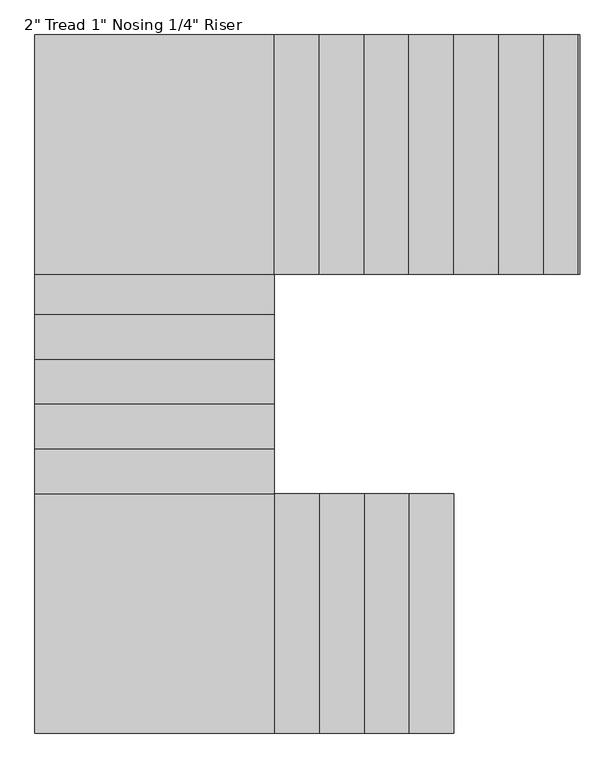
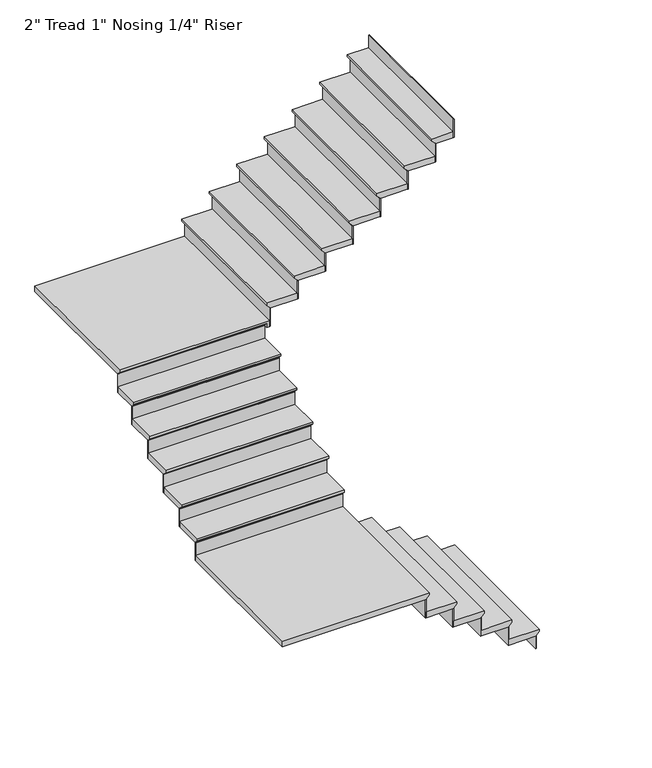
"""IFC4 building model written with IfcOpenShell, lengths in millimetres: stair flight geometry."""

from ifc_helpers import new_model, si_unit, origin, place, context, project, spatial, faceted_brep, source, transform, mapped, element, save


def stair_flight_d9589ae6(model_context):
    return source(origin(), model_context, "Body", "Brep", [
        faceted_brep([(-2683.1105391, -1521.8373761, 12790.5710526), (-2683.1105391, -1521.8373761, 12809.6210526), (-2683.1105391, -2741.0373761, 12809.6210526), (-2683.1105391, -2741.0373761, 12790.5710526), (-2708.5105391, -1521.8373761, 12765.1710526), (-2708.5105391, -2741.0373761, 12765.1710526), (-2937.1105391, -1521.8373761, 12809.6210526), (-2937.1105391, -2741.0373761, 12809.6210526), (-2708.5105391, -2741.0373761, 12758.8210526), (-2937.1105391, -2741.0373761, 12758.8210526), (-2937.1105391, -1521.8373761, 12758.8210526), (-2708.5105391, -1521.8373761, 12758.8210526)], [[[0, 1, 2, 3]], [[4, 0, 3, 5]], [[2, 1, 6, 7]], [[8, 9, 10, 11]], [[2, 7, 9, 8, 5, 3]], [[8, 11, 4, 5]], [[6, 1, 0, 4, 11, 10]], [[7, 6, 10, 9]]]),
        faceted_brep([(-2708.5105391, -1521.8373761, 12758.8210526), (-2708.5105391, -1521.8373761, 12649.2), (-2714.8605391, -1521.8373761, 12649.2), (-2714.8605391, -1521.8373761, 12758.8210526), (-2708.5105391, -2741.0373761, 12758.8210526), (-2714.8605391, -2741.0373761, 12758.8210526), (-2714.8605391, -2741.0373761, 12649.2), (-2708.5105391, -2741.0373761, 12649.2)], [[[0, 1, 2, 3]], [[4, 5, 6, 7]], [[1, 0, 4, 7]], [[2, 1, 7, 6]], [[3, 2, 6, 5]], [[0, 3, 5, 4]]]),
        faceted_brep([(-2937.1105391, -1521.8373761, 12919.2421053), (-2937.1105391, -1521.8373761, 12758.8210526), (-2943.4605391, -1521.8373761, 12758.8210526), (-2943.4605391, -1521.8373761, 12919.2421053), (-2937.1105391, -2741.0373761, 12919.2421053), (-2943.4605391, -2741.0373761, 12919.2421053), (-2943.4605391, -2741.0373761, 12758.8210526), (-2937.1105391, -2741.0373761, 12758.8210526)], [[[0, 1, 2, 3]], [[4, 5, 6, 7]], [[1, 0, 4, 7]], [[2, 1, 7, 6]], [[3, 2, 6, 5]], [[0, 3, 5, 4]]]),
        faceted_brep([(-2911.7105391, -2741.0373761, 12970.0421053), (-2911.7105391, -1521.8373761, 12970.0421053), (-3165.7105391, -1521.8373761, 12970.0421053), (-3165.7105391, -2741.0373761, 12970.0421053), (-2937.1105391, -2741.0373761, 12919.2421053), (-3165.7105391, -2741.0373761, 12919.2421053), (-3165.7105391, -1521.8373761, 12919.2421053), (-2937.1105391, -1521.8373761, 12919.2421053), (-2937.1105391, -2741.0373761, 12925.5921053), (-2911.7105391, -2741.0373761, 12950.9921053), (-2937.1105391, -1521.8373761, 12925.5921053), (-2911.7105391, -1521.8373761, 12950.9921053)], [[[0, 1, 2, 3]], [[4, 5, 6, 7]], [[0, 3, 5, 4, 8, 9]], [[4, 7, 10, 8]], [[2, 1, 11, 10, 7, 6]], [[3, 2, 6, 5]], [[11, 1, 0, 9]], [[10, 11, 9, 8]]]),
        faceted_brep([(-3165.7105391, -1521.8373761, 13079.6631579), (-3165.7105391, -1521.8373761, 12919.2421053), (-3172.0605391, -1521.8373761, 12919.2421053), (-3172.0605391, -1521.8373761, 13079.6631579), (-3165.7105391, -2741.0373761, 13079.6631579), (-3172.0605391, -2741.0373761, 13079.6631579), (-3172.0605391, -2741.0373761, 12919.2421053), (-3165.7105391, -2741.0373761, 12919.2421053)], [[[0, 1, 2, 3]], [[4, 5, 6, 7]], [[1, 0, 4, 7]], [[2, 1, 7, 6]], [[3, 2, 6, 5]], [[0, 3, 5, 4]]]),
        faceted_brep([(-3140.3105391, -2741.0373761, 13130.4631579), (-3140.3105391, -1521.8373761, 13130.4631579), (-3394.3105391, -1521.8373761, 13130.4631579), (-3394.3105391, -2741.0373761, 13130.4631579), (-3165.7105391, -2741.0373761, 13079.6631579), (-3394.3105391, -2741.0373761, 13079.6631579), (-3394.3105391, -1521.8373761, 13079.6631579), (-3165.7105391, -1521.8373761, 13079.6631579), (-3165.7105391, -2741.0373761, 13086.0131579), (-3140.3105391, -2741.0373761, 13111.4131579), (-3165.7105391, -1521.8373761, 13086.0131579), (-3140.3105391, -1521.8373761, 13111.4131579)], [[[0, 1, 2, 3]], [[4, 5, 6, 7]], [[0, 3, 5, 4, 8, 9]], [[4, 7, 10, 8]], [[2, 1, 11, 10, 7, 6]], [[3, 2, 6, 5]], [[11, 1, 0, 9]], [[10, 11, 9, 8]]]),
        faceted_brep([(-3394.3105391, -1521.8373761, 13240.0842105), (-3394.3105391, -1521.8373761, 13079.6631579), (-3400.6605391, -1521.8373761, 13079.6631579), (-3400.6605391, -1521.8373761, 13240.0842105), (-3394.3105391, -2741.0373761, 13240.0842105), (-3400.6605391, -2741.0373761, 13240.0842105), (-3400.6605391, -2741.0373761, 13079.6631579), (-3394.3105391, -2741.0373761, 13079.6631579)], [[[0, 1, 2, 3]], [[4, 5, 6, 7]], [[1, 0, 4, 7]], [[2, 1, 7, 6]], [[3, 2, 6, 5]], [[0, 3, 5, 4]]]),
        faceted_brep([(-3368.9105391, -2741.0373761, 13290.8842105), (-3368.9105391, -1521.8373761, 13290.8842105), (-3622.9105391, -1521.8373761, 13290.8842105), (-3622.9105391, -2741.0373761, 13290.8842105), (-3394.3105391, -2741.0373761, 13240.0842105), (-3622.9105391, -2741.0373761, 13240.0842105), (-3622.9105391, -1521.8373761, 13240.0842105), (-3394.3105391, -1521.8373761, 13240.0842105), (-3394.3105391, -2741.0373761, 13246.4342105), (-3368.9105391, -2741.0373761, 13271.8342105), (-3394.3105391, -1521.8373761, 13246.4342105), (-3368.9105391, -1521.8373761, 13271.8342105)], [[[0, 1, 2, 3]], [[4, 5, 6, 7]], [[0, 3, 5, 4, 8, 9]], [[4, 7, 10, 8]], [[2, 1, 11, 10, 7, 6]], [[3, 2, 6, 5]], [[11, 1, 0, 9]], [[10, 11, 9, 8]]]),
        faceted_brep([(-3622.9105391, -1521.8373761, 13400.5052632), (-3622.9105391, -1521.8373761, 13240.0842105), (-3629.2605391, -1521.8373761, 13240.0842105), (-3629.2605391, -1521.8373761, 13400.5052632), (-3622.9105391, -2741.0373761, 13400.5052632), (-3629.2605391, -2741.0373761, 13400.5052632), (-3629.2605391, -2741.0373761, 13240.0842105), (-3622.9105391, -2741.0373761, 13240.0842105)], [[[0, 1, 2, 3]], [[4, 5, 6, 7]], [[1, 0, 4, 7]], [[2, 1, 7, 6]], [[3, 2, 6, 5]], [[0, 3, 5, 4]]]),
        faceted_brep([(-4816.7105391, -1496.4373761, 13451.3052632), (-4816.7105391, -2741.0373761, 13451.3052632), (-3597.5105391, -2741.0373761, 13451.3052632), (-3597.5105391, -1496.4373761, 13451.3052632), (-4816.7105391, -2741.0373761, 13400.5052632), (-4816.7105391, -1496.4373761, 13400.5052632), (-3597.5105391, -1496.4373761, 13400.5052632), (-3597.5105391, -1521.8373761, 13400.5052632), (-3622.9105391, -1521.8373761, 13400.5052632), (-3622.9105391, -2741.0373761, 13400.5052632), (-3622.9105391, -2741.0373761, 13406.8552632), (-3597.5105391, -2741.0373761, 13432.2552632), (-3622.9105391, -1521.8373761, 13406.8552632), (-3597.5105391, -1521.8373761, 13432.2552632)], [[[0, 1, 2, 3]], [[4, 5, 6, 7, 8, 9]], [[1, 0, 5, 4]], [[2, 1, 4, 9, 10, 11]], [[9, 8, 12, 10]], [[8, 7, 13, 12]], [[3, 2, 11, 13, 7, 6]], [[0, 3, 6, 5]], [[11, 10, 12, 13]]]),
        faceted_brep([(-3597.5105391, -1496.4373761, 13560.9263158), (-3597.5105391, -1496.4373761, 13400.5052632), (-3597.5105391, -1490.0873761, 13400.5052632), (-3597.5105391, -1490.0873761, 13560.9263158), (-4816.7105391, -1496.4373761, 13560.9263158), (-4816.7105391, -1490.0873761, 13560.9263158), (-4816.7105391, -1490.0873761, 13400.5052632), (-4816.7105391, -1496.4373761, 13400.5052632)], [[[0, 1, 2, 3]], [[4, 5, 6, 7]], [[1, 0, 4, 7]], [[2, 1, 7, 6]], [[3, 2, 6, 5]], [[0, 3, 5, 4]]]),
        faceted_brep([(-4816.7105391, -1521.8373761, 13611.7263158), (-3597.5105391, -1521.8373761, 13611.7263158), (-3597.5105391, -1267.8373761, 13611.7263158), (-4816.7105391, -1267.8373761, 13611.7263158), (-4816.7105391, -1496.4373761, 13560.9263158), (-4816.7105391, -1267.8373761, 13560.9263158), (-3597.5105391, -1267.8373761, 13560.9263158), (-3597.5105391, -1496.4373761, 13560.9263158), (-4816.7105391, -1496.4373761, 13567.2763158), (-4816.7105391, -1521.8373761, 13592.6763158), (-3597.5105391, -1496.4373761, 13567.2763158), (-3597.5105391, -1521.8373761, 13592.6763158)], [[[0, 1, 2, 3]], [[4, 5, 6, 7]], [[0, 3, 5, 4, 8, 9]], [[4, 7, 10, 8]], [[2, 1, 11, 10, 7, 6]], [[3, 2, 6, 5]], [[11, 1, 0, 9]], [[10, 11, 9, 8]]]),
        faceted_brep([(-3597.5105391, -1267.8373761, 13721.3473684), (-3597.5105391, -1267.8373761, 13560.9263158), (-3597.5105391, -1261.4873761, 13560.9263158), (-3597.5105391, -1261.4873761, 13721.3473684), (-4816.7105391, -1267.8373761, 13721.3473684), (-4816.7105391, -1261.4873761, 13721.3473684), (-4816.7105391, -1261.4873761, 13560.9263158), (-4816.7105391, -1267.8373761, 13560.9263158)], [[[0, 1, 2, 3]], [[4, 5, 6, 7]], [[1, 0, 4, 7]], [[2, 1, 7, 6]], [[3, 2, 6, 5]], [[0, 3, 5, 4]]]),
        faceted_brep([(-4816.7105391, -1293.2373761, 13772.1473684), (-3597.5105391, -1293.2373761, 13772.1473684), (-3597.5105391, -1039.2373761, 13772.1473684), (-4816.7105391, -1039.2373761, 13772.1473684), (-4816.7105391, -1267.8373761, 13721.3473684), (-4816.7105391, -1039.2373761, 13721.3473684), (-3597.5105391, -1039.2373761, 13721.3473684), (-3597.5105391, -1267.8373761, 13721.3473684), (-4816.7105391, -1267.8373761, 13727.6973684), (-4816.7105391, -1293.2373761, 13753.0973684), (-3597.5105391, -1267.8373761, 13727.6973684), (-3597.5105391, -1293.2373761, 13753.0973684)], [[[0, 1, 2, 3]], [[4, 5, 6, 7]], [[0, 3, 5, 4, 8, 9]], [[4, 7, 10, 8]], [[2, 1, 11, 10, 7, 6]], [[3, 2, 6, 5]], [[11, 1, 0, 9]], [[10, 11, 9, 8]]]),
        faceted_brep([(-3597.5105391, -1039.2373761, 13881.7684211), (-3597.5105391, -1039.2373761, 13721.3473684), (-3597.5105391, -1032.8873761, 13721.3473684), (-3597.5105391, -1032.8873761, 13881.7684211), (-4816.7105391, -1039.2373761, 13881.7684211), (-4816.7105391, -1032.8873761, 13881.7684211), (-4816.7105391, -1032.8873761, 13721.3473684), (-4816.7105391, -1039.2373761, 13721.3473684)], [[[0, 1, 2, 3]], [[4, 5, 6, 7]], [[1, 0, 4, 7]], [[2, 1, 7, 6]], [[3, 2, 6, 5]], [[0, 3, 5, 4]]]),
        faceted_brep([(-4816.7105391, -1064.6373761, 13932.5684211), (-3597.5105391, -1064.6373761, 13932.5684211), (-3597.5105391, -810.6373761, 13932.5684211), (-4816.7105391, -810.6373761, 13932.5684211), (-4816.7105391, -1039.2373761, 13881.7684211), (-4816.7105391, -810.6373761, 13881.7684211), (-3597.5105391, -810.6373761, 13881.7684211), (-3597.5105391, -1039.2373761, 13881.7684211), (-4816.7105391, -1039.2373761, 13888.1184211), (-4816.7105391, -1064.6373761, 13913.5184211), (-3597.5105391, -1039.2373761, 13888.1184211), (-3597.5105391, -1064.6373761, 13913.5184211)], [[[0, 1, 2, 3]], [[4, 5, 6, 7]], [[0, 3, 5, 4, 8, 9]], [[4, 7, 10, 8]], [[2, 1, 11, 10, 7, 6]], [[3, 2, 6, 5]], [[11, 1, 0, 9]], [[10, 11, 9, 8]]]),
        faceted_brep([(-3597.5105391, -810.6373761, 14042.1894737), (-3597.5105391, -810.6373761, 13881.7684211), (-3597.5105391, -804.2873761, 13881.7684211), (-3597.5105391, -804.2873761, 14042.1894737), (-4816.7105391, -810.6373761, 14042.1894737), (-4816.7105391, -804.2873761, 14042.1894737), (-4816.7105391, -804.2873761, 13881.7684211), (-4816.7105391, -810.6373761, 13881.7684211)], [[[0, 1, 2, 3]], [[4, 5, 6, 7]], [[1, 0, 4, 7]], [[2, 1, 7, 6]], [[3, 2, 6, 5]], [[0, 3, 5, 4]]]),
        faceted_brep([(-4816.7105391, -836.0373761, 14092.9894737), (-3597.5105391, -836.0373761, 14092.9894737), (-3597.5105391, -582.0373761, 14092.9894737), (-4816.7105391, -582.0373761, 14092.9894737), (-4816.7105391, -810.6373761, 14042.1894737), (-4816.7105391, -582.0373761, 14042.1894737), (-3597.5105391, -582.0373761, 14042.1894737), (-3597.5105391, -810.6373761, 14042.1894737), (-4816.7105391, -810.6373761, 14048.5394737), (-4816.7105391, -836.0373761, 14073.9394737), (-3597.5105391, -810.6373761, 14048.5394737), (-3597.5105391, -836.0373761, 14073.9394737)], [[[0, 1, 2, 3]], [[4, 5, 6, 7]], [[0, 3, 5, 4, 8, 9]], [[4, 7, 10, 8]], [[2, 1, 11, 10, 7, 6]], [[3, 2, 6, 5]], [[11, 1, 0, 9]], [[10, 11, 9, 8]]]),
        faceted_brep([(-3597.5105391, -582.0373761, 14202.6105263), (-3597.5105391, -582.0373761, 14042.1894737), (-3597.5105391, -575.6873761, 14042.1894737), (-3597.5105391, -575.6873761, 14202.6105263), (-4816.7105391, -582.0373761, 14202.6105263), (-4816.7105391, -575.6873761, 14202.6105263), (-4816.7105391, -575.6873761, 14042.1894737), (-4816.7105391, -582.0373761, 14042.1894737)], [[[0, 1, 2, 3]], [[4, 5, 6, 7]], [[1, 0, 4, 7]], [[2, 1, 7, 6]], [[3, 2, 6, 5]], [[0, 3, 5, 4]]]),
        faceted_brep([(-4816.7105391, -607.4373761, 14253.4105263), (-3597.5105391, -607.4373761, 14253.4105263), (-3597.5105391, -378.8373761, 14253.4105263), (-4816.7105391, -378.8373761, 14253.4105263), (-4816.7105391, -582.0373761, 14202.6105263), (-4816.7105391, -378.8373761, 14202.6105263), (-3597.5105391, -378.8373761, 14202.6105263), (-3597.5105391, -582.0373761, 14202.6105263), (-4816.7105391, -582.0373761, 14208.9605263), (-4816.7105391, -607.4373761, 14234.3605263), (-3597.5105391, -582.0373761, 14208.9605263), (-3597.5105391, -607.4373761, 14234.3605263)], [[[0, 1, 2, 3]], [[4, 5, 6, 7]], [[0, 3, 5, 4, 8, 9]], [[4, 7, 10, 8]], [[2, 1, 11, 10, 7, 6]], [[3, 2, 6, 5]], [[11, 1, 0, 9]], [[10, 11, 9, 8]]]),
        faceted_brep([(-3597.5105391, -378.8373761, 14363.0315789), (-3597.5105391, -378.8373761, 14202.6105263), (-3597.5105391, -372.4873761, 14202.6105263), (-3597.5105391, -372.4873761, 14363.0315789), (-4816.7105391, -378.8373761, 14363.0315789), (-4816.7105391, -372.4873761, 14363.0315789), (-4816.7105391, -372.4873761, 14202.6105263), (-4816.7105391, -378.8373761, 14202.6105263)], [[[0, 1, 2, 3]], [[4, 5, 6, 7]], [[1, 0, 4, 7]], [[2, 1, 7, 6]], [[3, 2, 6, 5]], [[0, 3, 5, 4]]]),
        faceted_brep([(-3572.1105391, 814.9626239, 14413.8315789), (-4816.7105391, 814.9626239, 14413.8315789), (-4816.7105391, -404.2373761, 14413.8315789), (-3572.1105391, -404.2373761, 14413.8315789), (-4816.7105391, 814.9626239, 14363.0315789), (-3572.1105391, 814.9626239, 14363.0315789), (-3572.1105391, -404.2373761, 14363.0315789), (-3597.5105391, -404.2373761, 14363.0315789), (-3597.5105391, -378.8373761, 14363.0315789), (-4816.7105391, -378.8373761, 14363.0315789), (-4816.7105391, -378.8373761, 14369.3815789), (-4816.7105391, -404.2373761, 14394.7815789), (-3597.5105391, -378.8373761, 14369.3815789), (-3597.5105391, -404.2373761, 14394.7815789)], [[[0, 1, 2, 3]], [[4, 5, 6, 7, 8, 9]], [[1, 0, 5, 4]], [[2, 1, 4, 9, 10, 11]], [[9, 8, 12, 10]], [[8, 7, 13, 12]], [[3, 2, 11, 13, 7, 6]], [[0, 3, 6, 5]], [[11, 10, 12, 13]]]),
        faceted_brep([(-3572.1105391, -404.2373761, 14523.4526316), (-3572.1105391, -404.2373761, 14363.0315789), (-3565.7605391, -404.2373761, 14363.0315789), (-3565.7605391, -404.2373761, 14523.4526316), (-3572.1105391, 814.9626239, 14523.4526316), (-3565.7605391, 814.9626239, 14523.4526316), (-3565.7605391, 814.9626239, 14363.0315789), (-3572.1105391, 814.9626239, 14363.0315789)], [[[0, 1, 2, 3]], [[4, 5, 6, 7]], [[1, 0, 4, 7]], [[2, 1, 7, 6]], [[3, 2, 6, 5]], [[0, 3, 5, 4]]]),
        faceted_brep([(-3597.5105391, 814.9626239, 14574.2526316), (-3597.5105391, -404.2373761, 14574.2526316), (-3343.5105391, -404.2373761, 14574.2526316), (-3343.5105391, 814.9626239, 14574.2526316), (-3572.1105391, 814.9626239, 14523.4526316), (-3343.5105391, 814.9626239, 14523.4526316), (-3343.5105391, -404.2373761, 14523.4526316), (-3572.1105391, -404.2373761, 14523.4526316), (-3572.1105391, 814.9626239, 14529.8026316), (-3597.5105391, 814.9626239, 14555.2026316), (-3572.1105391, -404.2373761, 14529.8026316), (-3597.5105391, -404.2373761, 14555.2026316)], [[[0, 1, 2, 3]], [[4, 5, 6, 7]], [[0, 3, 5, 4, 8, 9]], [[4, 7, 10, 8]], [[2, 1, 11, 10, 7, 6]], [[3, 2, 6, 5]], [[11, 1, 0, 9]], [[10, 11, 9, 8]]]),
        faceted_brep([(-3343.5105391, -404.2373761, 14683.8736842), (-3343.5105391, -404.2373761, 14523.4526316), (-3337.1605391, -404.2373761, 14523.4526316), (-3337.1605391, -404.2373761, 14683.8736842), (-3343.5105391, 814.9626239, 14683.8736842), (-3337.1605391, 814.9626239, 14683.8736842), (-3337.1605391, 814.9626239, 14523.4526316), (-3343.5105391, 814.9626239, 14523.4526316)], [[[0, 1, 2, 3]], [[4, 5, 6, 7]], [[1, 0, 4, 7]], [[2, 1, 7, 6]], [[3, 2, 6, 5]], [[0, 3, 5, 4]]]),
        faceted_brep([(-3368.9105391, 814.9626239, 14734.6736842), (-3368.9105391, -404.2373761, 14734.6736842), (-3114.9105391, -404.2373761, 14734.6736842), (-3114.9105391, 814.9626239, 14734.6736842), (-3343.5105391, 814.9626239, 14683.8736842), (-3114.9105391, 814.9626239, 14683.8736842), (-3114.9105391, -404.2373761, 14683.8736842), (-3343.5105391, -404.2373761, 14683.8736842), (-3343.5105391, 814.9626239, 14690.2236842), (-3368.9105391, 814.9626239, 14715.6236842), (-3343.5105391, -404.2373761, 14690.2236842), (-3368.9105391, -404.2373761, 14715.6236842)], [[[0, 1, 2, 3]], [[4, 5, 6, 7]], [[0, 3, 5, 4, 8, 9]], [[4, 7, 10, 8]], [[2, 1, 11, 10, 7, 6]], [[3, 2, 6, 5]], [[11, 1, 0, 9]], [[10, 11, 9, 8]]]),
        faceted_brep([(-3114.9105391, -404.2373761, 14844.2947368), (-3114.9105391, -404.2373761, 14683.8736842), (-3108.5605391, -404.2373761, 14683.8736842), (-3108.5605391, -404.2373761, 14844.2947368), (-3114.9105391, 814.9626239, 14844.2947368), (-3108.5605391, 814.9626239, 14844.2947368), (-3108.5605391, 814.9626239, 14683.8736842), (-3114.9105391, 814.9626239, 14683.8736842)], [[[0, 1, 2, 3]], [[4, 5, 6, 7]], [[1, 0, 4, 7]], [[2, 1, 7, 6]], [[3, 2, 6, 5]], [[0, 3, 5, 4]]]),
        faceted_brep([(-3140.3105391, 814.9626239, 14895.0947368), (-3140.3105391, -404.2373761, 14895.0947368), (-2886.3105391, -404.2373761, 14895.0947368), (-2886.3105391, 814.9626239, 14895.0947368), (-3114.9105391, 814.9626239, 14844.2947368), (-2886.3105391, 814.9626239, 14844.2947368), (-2886.3105391, -404.2373761, 14844.2947368), (-3114.9105391, -404.2373761, 14844.2947368), (-3114.9105391, 814.9626239, 14850.6447368), (-3140.3105391, 814.9626239, 14876.0447368), (-3114.9105391, -404.2373761, 14850.6447368), (-3140.3105391, -404.2373761, 14876.0447368)], [[[0, 1, 2, 3]], [[4, 5, 6, 7]], [[0, 3, 5, 4, 8, 9]], [[4, 7, 10, 8]], [[2, 1, 11, 10, 7, 6]], [[3, 2, 6, 5]], [[11, 1, 0, 9]], [[10, 11, 9, 8]]]),
        faceted_brep([(-2886.3105391, -404.2373761, 15004.7157895), (-2886.3105391, -404.2373761, 14844.2947368), (-2879.9605391, -404.2373761, 14844.2947368), (-2879.9605391, -404.2373761, 15004.7157895), (-2886.3105391, 814.9626239, 15004.7157895), (-2879.9605391, 814.9626239, 15004.7157895), (-2879.9605391, 814.9626239, 14844.2947368), (-2886.3105391, 814.9626239, 14844.2947368)], [[[0, 1, 2, 3]], [[4, 5, 6, 7]], [[1, 0, 4, 7]], [[2, 1, 7, 6]], [[3, 2, 6, 5]], [[0, 3, 5, 4]]]),
        faceted_brep([(-2911.7105391, 814.9626239, 15055.5157895), (-2911.7105391, -404.2373761, 15055.5157895), (-2657.7105391, -404.2373761, 15055.5157895), (-2657.7105391, 814.9626239, 15055.5157895), (-2886.3105391, 814.9626239, 15004.7157895), (-2657.7105391, 814.9626239, 15004.7157895), (-2657.7105391, -404.2373761, 15004.7157895), (-2886.3105391, -404.2373761, 15004.7157895), (-2886.3105391, 814.9626239, 15011.0657895), (-2911.7105391, 814.9626239, 15036.4657895), (-2886.3105391, -404.2373761, 15011.0657895), (-2911.7105391, -404.2373761, 15036.4657895)], [[[0, 1, 2, 3]], [[4, 5, 6, 7]], [[0, 3, 5, 4, 8, 9]], [[4, 7, 10, 8]], [[2, 1, 11, 10, 7, 6]], [[3, 2, 6, 5]], [[11, 1, 0, 9]], [[10, 11, 9, 8]]]),
        faceted_brep([(-2657.7105391, -404.2373761, 15165.1368421), (-2657.7105391, -404.2373761, 15004.7157895), (-2651.3605391, -404.2373761, 15004.7157895), (-2651.3605391, -404.2373761, 15165.1368421), (-2657.7105391, 814.9626239, 15165.1368421), (-2651.3605391, 814.9626239, 15165.1368421), (-2651.3605391, 814.9626239, 15004.7157895), (-2657.7105391, 814.9626239, 15004.7157895)], [[[0, 1, 2, 3]], [[4, 5, 6, 7]], [[1, 0, 4, 7]], [[2, 1, 7, 6]], [[3, 2, 6, 5]], [[0, 3, 5, 4]]]),
        faceted_brep([(-2683.1105391, 814.9626239, 15215.9368421), (-2683.1105391, -404.2373761, 15215.9368421), (-2429.1105391, -404.2373761, 15215.9368421), (-2429.1105391, 814.9626239, 15215.9368421), (-2657.7105391, 814.9626239, 15165.1368421), (-2429.1105391, 814.9626239, 15165.1368421), (-2429.1105391, -404.2373761, 15165.1368421), (-2657.7105391, -404.2373761, 15165.1368421), (-2657.7105391, 814.9626239, 15171.4868421), (-2683.1105391, 814.9626239, 15196.8868421), (-2657.7105391, -404.2373761, 15171.4868421), (-2683.1105391, -404.2373761, 15196.8868421)], [[[0, 1, 2, 3]], [[4, 5, 6, 7]], [[0, 3, 5, 4, 8, 9]], [[4, 7, 10, 8]], [[2, 1, 11, 10, 7, 6]], [[3, 2, 6, 5]], [[11, 1, 0, 9]], [[10, 11, 9, 8]]]),
        faceted_brep([(-2429.1105391, -404.2373761, 15325.5578947), (-2429.1105391, -404.2373761, 15165.1368421), (-2422.7605391, -404.2373761, 15165.1368421), (-2422.7605391, -404.2373761, 15325.5578947), (-2429.1105391, 814.9626239, 15325.5578947), (-2422.7605391, 814.9626239, 15325.5578947), (-2422.7605391, 814.9626239, 15165.1368421), (-2429.1105391, 814.9626239, 15165.1368421)], [[[0, 1, 2, 3]], [[4, 5, 6, 7]], [[1, 0, 4, 7]], [[2, 1, 7, 6]], [[3, 2, 6, 5]], [[0, 3, 5, 4]]]),
        faceted_brep([(-2454.5105391, 814.9626239, 15376.3578947), (-2454.5105391, -404.2373761, 15376.3578947), (-2200.5105391, -404.2373761, 15376.3578947), (-2200.5105391, 814.9626239, 15376.3578947), (-2429.1105391, 814.9626239, 15325.5578947), (-2200.5105391, 814.9626239, 15325.5578947), (-2200.5105391, -404.2373761, 15325.5578947), (-2429.1105391, -404.2373761, 15325.5578947), (-2429.1105391, 814.9626239, 15331.9078947), (-2454.5105391, 814.9626239, 15357.3078947), (-2429.1105391, -404.2373761, 15331.9078947), (-2454.5105391, -404.2373761, 15357.3078947)], [[[0, 1, 2, 3]], [[4, 5, 6, 7]], [[0, 3, 5, 4, 8, 9]], [[4, 7, 10, 8]], [[2, 1, 11, 10, 7, 6]], [[3, 2, 6, 5]], [[11, 1, 0, 9]], [[10, 11, 9, 8]]]),
        faceted_brep([(-2200.5105391, -404.2373761, 15485.9789474), (-2200.5105391, -404.2373761, 15325.5578947), (-2194.1605391, -404.2373761, 15325.5578947), (-2194.1605391, -404.2373761, 15485.9789474), (-2200.5105391, 814.9626239, 15485.9789474), (-2194.1605391, 814.9626239, 15485.9789474), (-2194.1605391, 814.9626239, 15325.5578947), (-2200.5105391, 814.9626239, 15325.5578947)], [[[0, 1, 2, 3]], [[4, 5, 6, 7]], [[1, 0, 4, 7]], [[2, 1, 7, 6]], [[3, 2, 6, 5]], [[0, 3, 5, 4]]]),
        faceted_brep([(-2048.1105391, -404.2373761, 15646.4), (-2048.1105391, -404.2373761, 15485.9789474), (-2041.7605391, -404.2373761, 15485.9789474), (-2041.7605391, -404.2373761, 15646.4), (-2048.1105391, 814.9626239, 15646.4), (-2041.7605391, 814.9626239, 15646.4), (-2041.7605391, 814.9626239, 15485.9789474), (-2048.1105391, 814.9626239, 15485.9789474)], [[[0, 1, 2, 3]], [[4, 5, 6, 7]], [[1, 0, 4, 7]], [[2, 1, 7, 6]], [[3, 2, 6, 5]], [[0, 3, 5, 4]]]),
        faceted_brep([(-2225.9105391, 814.9626239, 15536.7789474), (-2225.9105391, -404.2373761, 15536.7789474), (-2048.1105391, -404.2373761, 15536.7789474), (-2048.1105391, 814.9626239, 15536.7789474), (-2200.5105391, 814.9626239, 15485.9789474), (-2048.1105391, 814.9626239, 15485.9789474), (-2048.1105391, -404.2373761, 15485.9789474), (-2200.5105391, -404.2373761, 15485.9789474), (-2200.5105391, 814.9626239, 15492.3289474), (-2225.9105391, 814.9626239, 15517.7289474), (-2200.5105391, -404.2373761, 15492.3289474), (-2225.9105391, -404.2373761, 15517.7289474)], [[[0, 1, 2, 3]], [[4, 5, 6, 7]], [[0, 3, 5, 4, 8, 9]], [[4, 7, 10, 8]], [[2, 1, 11, 10, 7, 6]], [[3, 2, 6, 5]], [[11, 1, 0, 9]], [[10, 11, 9, 8]]]),
    ])


if __name__ == "__main__":
    model = new_model("IFC4")
    model_context = context("Model", 3, world=origin())
    ifc_project = project(units=[si_unit("LENGTHUNIT", "METRE", prefix="MILLI")], contexts=[model_context])
    site = spatial("IfcSite", under=ifc_project)
    building = spatial("IfcBuilding", under=site)
    placement = place(None, origin())
    stair_flight_shape = stair_flight_d9589ae6(model_context)
    element("IfcStairFlight", 1, ObjectType="2\" Tread 1\" Nosing 1/4\" Riser", at=placement, inside=building, context=model_context, shape_type="MappedRepresentation", body=[
        mapped(stair_flight_shape, transform((0.0, 0.0, 0.0), x_axis=(1.0, 0.0, 0.0), y_axis=(0.0, 1.0, 0.0), z_axis=(0.0, 0.0, 1.0))),
    ])
    save(model, "model.ifc")
